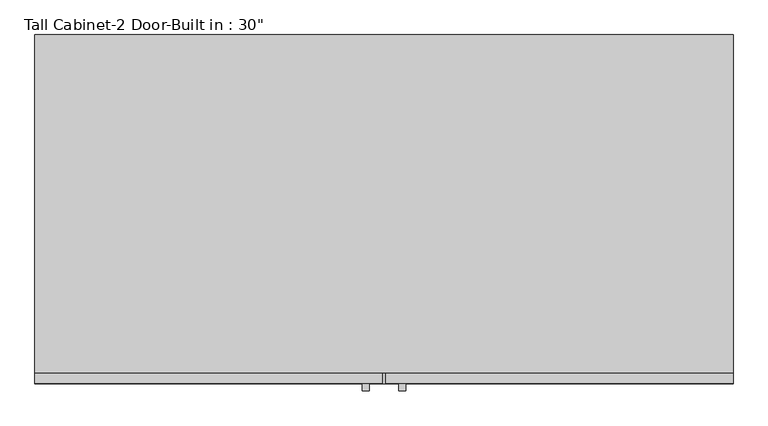
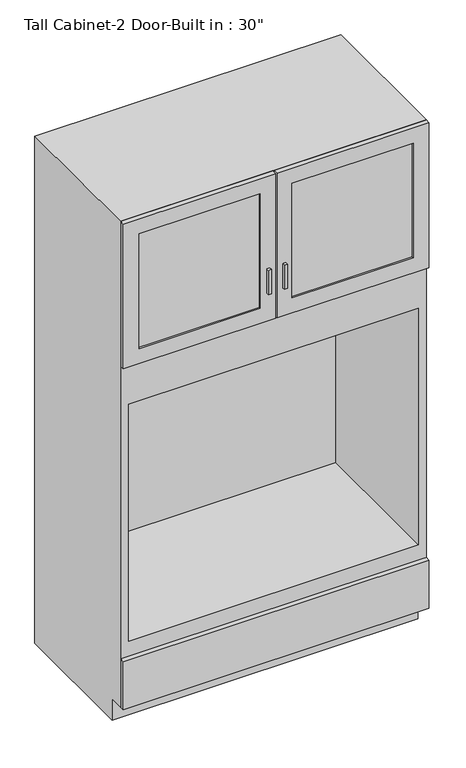
"""IFC4 building model written with IfcOpenShell, lengths in millimetres: furniture geometry."""

from ifc_helpers import new_model, si_unit, frame, origin, place, context, project, spatial, polyline, outline, extrude, faceted_brep, source, transform, mapped, element, save


def furniture_4aee2c20(model_context):
    return source(origin(), model_context, "Body", "SolidModel", [
        faceted_brep([(628.3377049, -590.55, 90.4875), (628.3377049, -590.55, 2135.1875), (-590.8622951, -590.55, 2135.1875), (-590.8622951, -590.55, 90.4875), (-571.8122951, -590.55, 2116.1375), (609.2877049, -590.55, 2116.1375), (609.2877049, -590.55, 1525.5875), (-571.8122951, -590.55, 1525.5875), (596.5877049, -590.55, 357.1875), (-559.1122951, -590.55, 357.1875), (-559.1122951, -590.55, 1354.1375), (596.5877049, -590.55, 1354.1375), (-590.8622951, 0.0, 2135.1875), (628.3377049, 0.0, 2135.1875), (628.3377049, 0.0, 0.0), (-590.8622951, 0.0, 0.0), (628.3377049, -533.4, 90.4875), (628.3377049, -533.4, 0.0), (-590.8622951, -533.4, 0.0), (-590.8622951, -533.4, 90.4875), (609.2877049, -19.05, 2116.1375), (609.2877049, -19.05, 1525.5875), (-571.8122951, -19.05, 1525.5875), (-571.8122951, -19.05, 2116.1375), (596.5877049, -19.05, 357.1875), (-559.1122951, -19.05, 357.1875), (-559.1122951, -19.05, 1354.1375), (596.5877049, -19.05, 1354.1375)], [[[0, 1, 2, 3], [4, 5, 6, 7], [8, 9, 10, 11]], [[12, 13, 14, 15]], [[1, 0, 16, 17, 14, 13]], [[2, 1, 13, 12]], [[3, 2, 12, 15, 18, 19]], [[0, 3, 19, 16]], [[6, 5, 20, 21]], [[4, 7, 22, 23]], [[5, 4, 23, 20]], [[14, 17, 18, 15]], [[18, 17, 16, 19]], [[7, 6, 21, 22]], [[9, 8, 24, 25]], [[10, 9, 25, 26]], [[11, 10, 26, 27]], [[8, 11, 27, 24]], [[21, 20, 23, 22]], [[25, 24, 27, 26]]]),
        extrude(outline(polyline([(628.3377049, -609.6), (-590.8622951, -609.6), (-590.8622951, -590.55), (628.3377049, -590.55), (628.3377049, -609.6)])), frame((0.0, 0.0, 90.4875), z_axis=(0.0, 0.0, 1.0), x_axis=(1.0, 0.0, 0.0)), (0.0, 0.0, 1.0), 203.2),
        extrude(outline(polyline([(2135.1875, 15.5627049), (2135.1875, -590.8622951), (1525.5875, -590.8622951), (1525.5875, 15.5627049), (2135.1875, 15.5627049)]), holes=[polyline([(2071.6875, -44.7622951), (1589.0875, -44.7622951), (1589.0875, -527.3622951), (2071.6875, -527.3622951), (2071.6875, -44.7622951)])]), frame((0.0, -609.6, 0.0), z_axis=(0.0, 1.0, 0.0), x_axis=(0.0, 0.0, 1.0)), (0.0, 0.0, 1.0), 19.05),
        extrude(outline(polyline([(2135.1875, 21.9127049), (1525.5875, 21.9127049), (1525.5875, 628.3377049), (2135.1875, 628.3377049), (2135.1875, 21.9127049)]), holes=[polyline([(2071.6875, 564.8377049), (1589.0875, 564.8377049), (1589.0875, 82.2377049), (2071.6875, 82.2377049), (2071.6875, 564.8377049)])]), frame((0.0, -609.6, 0.0), z_axis=(0.0, 1.0, 0.0), x_axis=(0.0, 0.0, 1.0)), (0.0, 0.0, 1.0), 19.05),
        extrude(outline(polyline([(628.3377049, -609.6), (-590.8622951, -609.6), (-590.8622951, -590.55), (628.3377049, -590.55), (628.3377049, -609.6)])), frame((0.0, 0.0, 90.4875), z_axis=(0.0, 0.0, 1.0), x_axis=(1.0, 0.0, 0.0)), (0.0, 0.0, 1.0), 203.2),
        extrude(outline(polyline([(-6.6622951, -622.3), (-19.1945267, -622.3), (-19.1945267, -609.6), (-6.6622951, -609.6), (-6.6622951, -622.3)])), frame((0.0, 0.0, 1645.6417867), z_axis=(0.0, 0.0, 1.0), x_axis=(1.0, 0.0, 0.0)), (0.0, 0.0, 1.0), 101.6),
        extrude(outline(polyline([(56.6699365, -622.3), (44.1377049, -622.3), (44.1377049, -609.6), (56.6699365, -609.6), (56.6699365, -622.3)])), frame((0.0, 0.0, 1645.6417867), z_axis=(0.0, 0.0, 1.0), x_axis=(1.0, 0.0, 0.0)), (0.0, 0.0, 1.0), 101.6),
        extrude(outline(polyline([(-44.7622951, -603.25), (-527.3622951, -603.25), (-527.3622951, -596.9), (-44.7622951, -596.9), (-44.7622951, -603.25)])), frame((0.0, 0.0, 1589.0875), z_axis=(0.0, 0.0, 1.0), x_axis=(1.0, 0.0, 0.0)), (0.0, 0.0, 1.0), 482.6),
        extrude(outline(polyline([(564.8377049, -603.25), (82.2377049, -603.25), (82.2377049, -596.9), (564.8377049, -596.9), (564.8377049, -603.25)])), frame((0.0, 0.0, 1589.0875), z_axis=(0.0, 0.0, 1.0), x_axis=(1.0, 0.0, 0.0)), (0.0, 0.0, 1.0), 482.6),
    ])


if __name__ == "__main__":
    model = new_model("IFC4")
    model_context = context("Model", 3, world=origin())
    ifc_project = project(units=[si_unit("LENGTHUNIT", "METRE", prefix="MILLI")], contexts=[model_context])
    site = spatial("IfcSite", under=ifc_project)
    building = spatial("IfcBuilding", under=site)
    placement = place(None, origin())
    furniture_shape = furniture_4aee2c20(model_context)
    element("IfcFurniture", 1, ObjectType="Tall Cabinet-2 Door-Built in : 30\"", at=placement, inside=building, context=model_context, shape_type="MappedRepresentation", body=[
        mapped(furniture_shape, transform((0.0, 0.0, 0.0), x_axis=(1.0, 0.0, 0.0), y_axis=(0.0, 1.0, 0.0), z_axis=(0.0, 0.0, 1.0))),
    ])
    save(model, "model.ifc")

# Revit data of these elements
# Type "Tall Cabinet-2 Door-Built in : 30\""
#   Assembly Code = "C1030410"
#   Height = 7' - 0"
#   Depth = 2' - 0"
#   Height-Base of Built-in = 1' - 2"
#   Height-Built-in = 3' - 3 1/4"
#   Height-Upper Cabinet = 2' - 0"
#   Toe Depth = 0' - 3"
#   Toe Height = 0' - 3 1/2"
#   Width = 4' - 0"
#   Cabinet Material = none
#   Door/Drawer Material = none
#   Handle Material = Cabinets - Handles
#   Panel Material = Glass
#   Default Elevation = 0
#   Type Comments = ""
# Element 1 (IfcFurniture, "Tall Cabinet-2 Door-Built in : 30\"")
#   Materials on its faces: "Cabinets", "Cabinets - Handles", "Glass"
# Materials
#   "Cabinets - Handles": class "Metal", colour RGB 57 57 57, transparency 0
#   "Glass": class "Glass", colour RGB 0 128 192, transparency 0.75, Description = "Soda Lime Glass", Cost = 0
#   "Cabinets": colour RGB 249 249 249, transparency 0
